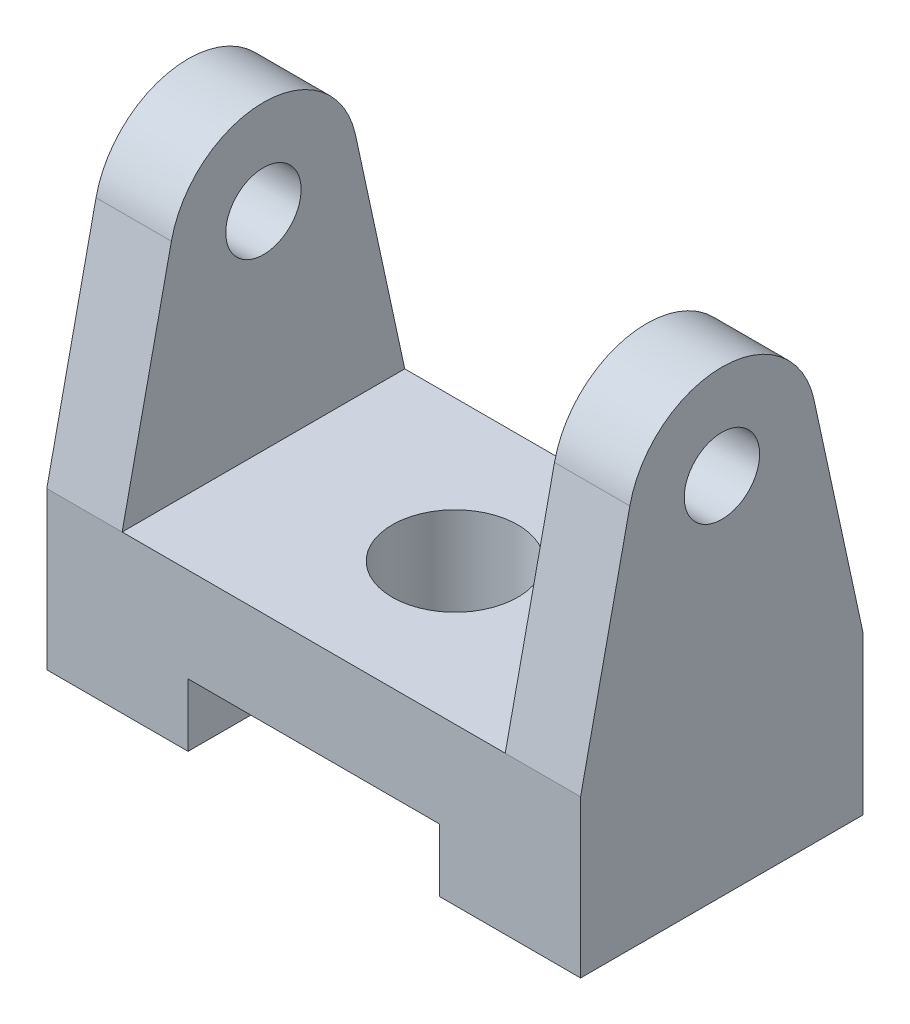
ISO-10303-21;
HEADER;
FILE_DESCRIPTION(('STEP AP214'),'2;1');
FILE_NAME('part.step','',(''),(''),'','','');
FILE_SCHEMA(('AUTOMOTIVE_DESIGN { 1 0 10303 214 1 1 1 1 }'));
ENDSEC;
DATA;
#1=APPLICATION_CONTEXT('core data for automotive mechanical design processes');
#2=APPLICATION_PROTOCOL_DEFINITION('international standard','automotive_design',2000,#1);
#3=PRODUCT_CONTEXT('',#1,'mechanical');
#4=PRODUCT('Part','Part','',(#3));
#5=PRODUCT_RELATED_PRODUCT_CATEGORY('part','',(#4));
#6=PRODUCT_DEFINITION_FORMATION('','',#4);
#7=PRODUCT_DEFINITION_CONTEXT('part definition',#1,'design');
#8=PRODUCT_DEFINITION('design','',#6,#7);
#9=PRODUCT_DEFINITION_SHAPE('','',#8);
#10=(LENGTH_UNIT() NAMED_UNIT(*) SI_UNIT(.MILLI.,.METRE.));
#11=(NAMED_UNIT(*) PLANE_ANGLE_UNIT() SI_UNIT($,.RADIAN.));
#12=(NAMED_UNIT(*) SI_UNIT($,.STERADIAN.) SOLID_ANGLE_UNIT());
#13=UNCERTAINTY_MEASURE_WITH_UNIT(LENGTH_MEASURE(1.E-05),#10,'distance_accuracy_value','');
#14=(GEOMETRIC_REPRESENTATION_CONTEXT(3) GLOBAL_UNCERTAINTY_ASSIGNED_CONTEXT((#13)) GLOBAL_UNIT_ASSIGNED_CONTEXT((#10,
#11,#12)) REPRESENTATION_CONTEXT('',''));
#15=CARTESIAN_POINT('',(0.,0.,0.));
#16=DIRECTION('',(0.,0.,1.));
#17=DIRECTION('',(1.,0.,0.));
#18=AXIS2_PLACEMENT_3D('',#15,#16,#17);
#19=CARTESIAN_POINT('',(-42.5,25.,45.));
#20=DIRECTION('',(0.,-1.,0.));
#21=DIRECTION('',(0.,0.,-1.));
#22=AXIS2_PLACEMENT_3D('',#19,#20,#21);
#23=PLANE('',#22);
#24=CARTESIAN_POINT('',(0.,25.,22.5));
#25=DIRECTION('',(0.,1.,0.));
#26=DIRECTION('',(0.,0.,1.));
#27=AXIS2_PLACEMENT_3D('',#24,#25,#26);
#28=CIRCLE('',#27,10.);
#29=CARTESIAN_POINT('',(0.,25.,32.5));
#30=VERTEX_POINT('',#29);
#31=EDGE_CURVE('E212',#30,#30,#28,.T.);
#32=ORIENTED_EDGE('',*,*,#31,.F.);
#33=EDGE_LOOP('',(#32));
#34=FACE_BOUND('',#33,.T.);
#35=DIRECTION('',(0.,0.,-1.));
#36=VECTOR('',#35,1.);
#37=CARTESIAN_POINT('',(30.5,25.,45.));
#38=LINE('',#37,#36);
#39=CARTESIAN_POINT('',(30.5,25.,45.));
#40=VERTEX_POINT('',#39);
#41=CARTESIAN_POINT('',(30.5,25.,0.));
#42=VERTEX_POINT('',#41);
#43=EDGE_CURVE('E170',#40,#42,#38,.T.);
#44=ORIENTED_EDGE('',*,*,#43,.T.);
#45=DIRECTION('',(-1.,0.,0.));
#46=VECTOR('',#45,1.);
#47=CARTESIAN_POINT('',(-42.5,25.,0.));
#48=LINE('',#47,#46);
#49=CARTESIAN_POINT('',(-30.5,25.,0.));
#50=VERTEX_POINT('',#49);
#51=EDGE_CURVE('E245',#42,#50,#48,.T.);
#52=ORIENTED_EDGE('',*,*,#51,.T.);
#53=DIRECTION('',(0.,0.,1.));
#54=VECTOR('',#53,1.);
#55=CARTESIAN_POINT('',(-30.5,25.,0.));
#56=LINE('',#55,#54);
#57=CARTESIAN_POINT('',(-30.5,25.,45.));
#58=VERTEX_POINT('',#57);
#59=EDGE_CURVE('E192',#50,#58,#56,.T.);
#60=ORIENTED_EDGE('',*,*,#59,.T.);
#61=DIRECTION('',(-1.,0.,0.));
#62=VECTOR('',#61,1.);
#63=CARTESIAN_POINT('',(-42.5,25.,45.));
#64=LINE('',#63,#62);
#65=EDGE_CURVE('E58',#40,#58,#64,.T.);
#66=ORIENTED_EDGE('',*,*,#65,.F.);
#67=EDGE_LOOP('',(#44,#52,#60,#66));
#68=FACE_BOUND('',#67,.T.);
#69=ADVANCED_FACE('F44',(#34,#68),#23,.F.);
#70=CARTESIAN_POINT('',(-42.5,0.,45.));
#71=DIRECTION('',(1.,0.,0.));
#72=DIRECTION('',(0.,0.,-1.));
#73=AXIS2_PLACEMENT_3D('',#70,#71,#72);
#74=PLANE('',#73);
#75=DIRECTION('',(0.,-1.,0.));
#76=VECTOR('',#75,1.);
#77=CARTESIAN_POINT('',(-42.5,0.,0.));
#78=LINE('',#77,#76);
#79=CARTESIAN_POINT('',(-42.5,25.,0.));
#80=VERTEX_POINT('',#79);
#81=CARTESIAN_POINT('',(-42.5,0.,0.));
#82=VERTEX_POINT('',#81);
#83=EDGE_CURVE('E241',#80,#82,#78,.T.);
#84=ORIENTED_EDGE('',*,*,#83,.T.);
#85=DIRECTION('',(0.,0.,-1.));
#86=VECTOR('',#85,1.);
#87=CARTESIAN_POINT('',(-42.5,0.,45.));
#88=LINE('',#87,#86);
#89=CARTESIAN_POINT('',(-42.5,0.,45.));
#90=VERTEX_POINT('',#89);
#91=EDGE_CURVE('E11',#90,#82,#88,.T.);
#92=ORIENTED_EDGE('',*,*,#91,.F.);
#93=DIRECTION('',(0.,-1.,0.));
#94=VECTOR('',#93,1.);
#95=CARTESIAN_POINT('',(-42.5,0.,45.));
#96=LINE('',#95,#94);
#97=CARTESIAN_POINT('',(-42.5,25.,45.));
#98=VERTEX_POINT('',#97);
#99=EDGE_CURVE('E221',#98,#90,#96,.T.);
#100=ORIENTED_EDGE('',*,*,#99,.F.);
#101=DIRECTION('',(0.,0.977312211406396,-0.211803780504361));
#102=VECTOR('',#101,1.);
#103=CARTESIAN_POINT('',(-42.5,25.,45.));
#104=LINE('',#103,#102);
#105=CARTESIAN_POINT('',(-42.5,61.1770567075654,37.159683171096));
#106=VERTEX_POINT('',#105);
#107=EDGE_CURVE('E210',#98,#106,#104,.T.);
#108=ORIENTED_EDGE('',*,*,#107,.T.);
#109=CARTESIAN_POINT('',(-42.5,58.,22.5));
#110=DIRECTION('',(-1.,0.,0.));
#111=DIRECTION('',(0.,0.,1.));
#112=AXIS2_PLACEMENT_3D('',#109,#110,#111);
#113=CIRCLE('',#112,15.);
#114=CARTESIAN_POINT('',(-42.5,61.1770567075654,7.84031682890406));
#115=VERTEX_POINT('',#114);
#116=EDGE_CURVE('E198',#106,#115,#113,.T.);
#117=ORIENTED_EDGE('',*,*,#116,.T.);
#118=DIRECTION('',(0.,-0.977312211406396,-0.211803780504361));
#119=VECTOR('',#118,1.);
#120=CARTESIAN_POINT('',(-42.5,25.,0.));
#121=LINE('',#120,#119);
#122=EDGE_CURVE('E188',#115,#80,#121,.T.);
#123=ORIENTED_EDGE('',*,*,#122,.T.);
#124=EDGE_LOOP('',(#84,#92,#100,#108,#117,#123));
#125=FACE_BOUND('',#124,.T.);
#126=CARTESIAN_POINT('',(-42.5,58.,22.5));
#127=DIRECTION('',(-1.,0.,0.));
#128=DIRECTION('',(0.,0.,1.));
#129=AXIS2_PLACEMENT_3D('',#126,#127,#128);
#130=CIRCLE('',#129,6.00000000000001);
#131=CARTESIAN_POINT('',(-42.5,58.,28.5));
#132=VERTEX_POINT('',#131);
#133=EDGE_CURVE('E184',#132,#132,#130,.T.);
#134=ORIENTED_EDGE('',*,*,#133,.F.);
#135=EDGE_LOOP('',(#134));
#136=FACE_BOUND('',#135,.T.);
#137=ADVANCED_FACE('F297',(#125,#136),#74,.F.);
#138=CARTESIAN_POINT('',(-20.,0.,45.));
#139=DIRECTION('',(0.,1.,0.));
#140=DIRECTION('',(0.,0.,1.));
#141=AXIS2_PLACEMENT_3D('',#138,#139,#140);
#142=PLANE('',#141);
#143=DIRECTION('',(1.,0.,0.));
#144=VECTOR('',#143,1.);
#145=CARTESIAN_POINT('',(-20.,0.,0.));
#146=LINE('',#145,#144);
#147=CARTESIAN_POINT('',(-20.,0.,0.));
#148=VERTEX_POINT('',#147);
#149=EDGE_CURVE('E242',#82,#148,#146,.T.);
#150=ORIENTED_EDGE('',*,*,#149,.T.);
#151=DIRECTION('',(0.,0.,-1.));
#152=VECTOR('',#151,1.);
#153=CARTESIAN_POINT('',(-20.,0.,45.));
#154=LINE('',#153,#152);
#155=CARTESIAN_POINT('',(-20.,0.,45.));
#156=VERTEX_POINT('',#155);
#157=EDGE_CURVE('E52',#156,#148,#154,.T.);
#158=ORIENTED_EDGE('',*,*,#157,.F.);
#159=DIRECTION('',(1.,0.,0.));
#160=VECTOR('',#159,1.);
#161=CARTESIAN_POINT('',(-20.,0.,45.));
#162=LINE('',#161,#160);
#163=EDGE_CURVE('E229',#90,#156,#162,.T.);
#164=ORIENTED_EDGE('',*,*,#163,.F.);
#165=ORIENTED_EDGE('',*,*,#91,.T.);
#166=EDGE_LOOP('',(#150,#158,#164,#165));
#167=FACE_BOUND('',#166,.T.);
#168=ADVANCED_FACE('F300',(#167),#142,.F.);
#169=CARTESIAN_POINT('',(-20.,10.,45.));
#170=DIRECTION('',(-1.,0.,0.));
#171=DIRECTION('',(0.,0.,1.));
#172=AXIS2_PLACEMENT_3D('',#169,#170,#171);
#173=PLANE('',#172);
#174=DIRECTION('',(0.,1.,0.));
#175=VECTOR('',#174,1.);
#176=CARTESIAN_POINT('',(-20.,10.,0.));
#177=LINE('',#176,#175);
#178=CARTESIAN_POINT('',(-20.,10.,0.));
#179=VERTEX_POINT('',#178);
#180=EDGE_CURVE('E250',#148,#179,#177,.T.);
#181=ORIENTED_EDGE('',*,*,#180,.T.);
#182=DIRECTION('',(0.,0.,-1.));
#183=VECTOR('',#182,1.);
#184=CARTESIAN_POINT('',(-20.,10.,45.));
#185=LINE('',#184,#183);
#186=CARTESIAN_POINT('',(-20.,10.,45.));
#187=VERTEX_POINT('',#186);
#188=EDGE_CURVE('E264',#187,#179,#185,.T.);
#189=ORIENTED_EDGE('',*,*,#188,.F.);
#190=DIRECTION('',(0.,1.,0.));
#191=VECTOR('',#190,1.);
#192=CARTESIAN_POINT('',(-20.,10.,45.));
#193=LINE('',#192,#191);
#194=EDGE_CURVE('E230',#156,#187,#193,.T.);
#195=ORIENTED_EDGE('',*,*,#194,.F.);
#196=ORIENTED_EDGE('',*,*,#157,.T.);
#197=EDGE_LOOP('',(#181,#189,#195,#196));
#198=FACE_BOUND('',#197,.T.);
#199=ADVANCED_FACE('F272',(#198),#173,.F.);
#200=CARTESIAN_POINT('',(20.,10.,45.));
#201=DIRECTION('',(0.,1.,0.));
#202=DIRECTION('',(0.,0.,1.));
#203=AXIS2_PLACEMENT_3D('',#200,#201,#202);
#204=PLANE('',#203);
#205=CARTESIAN_POINT('',(0.,10.,22.5));
#206=DIRECTION('',(0.,1.,0.));
#207=DIRECTION('',(0.,0.,1.));
#208=AXIS2_PLACEMENT_3D('',#205,#206,#207);
#209=CIRCLE('',#208,10.);
#210=CARTESIAN_POINT('',(0.,10.,32.5));
#211=VERTEX_POINT('',#210);
#212=EDGE_CURVE('E48',#211,#211,#209,.T.);
#213=ORIENTED_EDGE('',*,*,#212,.T.);
#214=EDGE_LOOP('',(#213));
#215=FACE_BOUND('',#214,.T.);
#216=DIRECTION('',(1.,0.,0.));
#217=VECTOR('',#216,1.);
#218=CARTESIAN_POINT('',(20.,10.,0.));
#219=LINE('',#218,#217);
#220=CARTESIAN_POINT('',(20.,10.,0.));
#221=VERTEX_POINT('',#220);
#222=EDGE_CURVE('E249',#179,#221,#219,.T.);
#223=ORIENTED_EDGE('',*,*,#222,.T.);
#224=DIRECTION('',(0.,0.,-1.));
#225=VECTOR('',#224,1.);
#226=CARTESIAN_POINT('',(20.,10.,45.));
#227=LINE('',#226,#225);
#228=CARTESIAN_POINT('',(20.,10.,45.));
#229=VERTEX_POINT('',#228);
#230=EDGE_CURVE('E265',#229,#221,#227,.T.);
#231=ORIENTED_EDGE('',*,*,#230,.F.);
#232=DIRECTION('',(1.,0.,0.));
#233=VECTOR('',#232,1.);
#234=CARTESIAN_POINT('',(20.,10.,45.));
#235=LINE('',#234,#233);
#236=EDGE_CURVE('E227',#187,#229,#235,.T.);
#237=ORIENTED_EDGE('',*,*,#236,.F.);
#238=ORIENTED_EDGE('',*,*,#188,.T.);
#239=EDGE_LOOP('',(#223,#231,#237,#238));
#240=FACE_BOUND('',#239,.T.);
#241=ADVANCED_FACE('F290',(#215,#240),#204,.F.);
#242=CARTESIAN_POINT('',(20.,0.,45.));
#243=DIRECTION('',(1.,0.,0.));
#244=DIRECTION('',(0.,0.,-1.));
#245=AXIS2_PLACEMENT_3D('',#242,#243,#244);
#246=PLANE('',#245);
#247=DIRECTION('',(0.,-1.,0.));
#248=VECTOR('',#247,1.);
#249=CARTESIAN_POINT('',(20.,0.,0.));
#250=LINE('',#249,#248);
#251=CARTESIAN_POINT('',(20.,0.,0.));
#252=VERTEX_POINT('',#251);
#253=EDGE_CURVE('E253',#221,#252,#250,.T.);
#254=ORIENTED_EDGE('',*,*,#253,.T.);
#255=DIRECTION('',(0.,0.,-1.));
#256=VECTOR('',#255,1.);
#257=CARTESIAN_POINT('',(20.,0.,45.));
#258=LINE('',#257,#256);
#259=CARTESIAN_POINT('',(20.,0.,45.));
#260=VERTEX_POINT('',#259);
#261=EDGE_CURVE('E259',#260,#252,#258,.T.);
#262=ORIENTED_EDGE('',*,*,#261,.F.);
#263=DIRECTION('',(0.,-1.,0.));
#264=VECTOR('',#263,1.);
#265=CARTESIAN_POINT('',(20.,0.,45.));
#266=LINE('',#265,#264);
#267=EDGE_CURVE('E235',#229,#260,#266,.T.);
#268=ORIENTED_EDGE('',*,*,#267,.F.);
#269=ORIENTED_EDGE('',*,*,#230,.T.);
#270=EDGE_LOOP('',(#254,#262,#268,#269));
#271=FACE_BOUND('',#270,.T.);
#272=ADVANCED_FACE('F292',(#271),#246,.F.);
#273=CARTESIAN_POINT('',(42.5,0.,45.));
#274=DIRECTION('',(0.,1.,0.));
#275=DIRECTION('',(0.,0.,1.));
#276=AXIS2_PLACEMENT_3D('',#273,#274,#275);
#277=PLANE('',#276);
#278=DIRECTION('',(1.,0.,0.));
#279=VECTOR('',#278,1.);
#280=CARTESIAN_POINT('',(42.5,0.,0.));
#281=LINE('',#280,#279);
#282=CARTESIAN_POINT('',(42.5,0.,0.));
#283=VERTEX_POINT('',#282);
#284=EDGE_CURVE('E251',#252,#283,#281,.T.);
#285=ORIENTED_EDGE('',*,*,#284,.T.);
#286=DIRECTION('',(0.,0.,-1.));
#287=VECTOR('',#286,1.);
#288=CARTESIAN_POINT('',(42.5,0.,45.));
#289=LINE('',#288,#287);
#290=CARTESIAN_POINT('',(42.5,0.,45.));
#291=VERTEX_POINT('',#290);
#292=EDGE_CURVE('E236',#291,#283,#289,.T.);
#293=ORIENTED_EDGE('',*,*,#292,.F.);
#294=DIRECTION('',(1.,0.,0.));
#295=VECTOR('',#294,1.);
#296=CARTESIAN_POINT('',(42.5,0.,45.));
#297=LINE('',#296,#295);
#298=EDGE_CURVE('E234',#260,#291,#297,.T.);
#299=ORIENTED_EDGE('',*,*,#298,.F.);
#300=ORIENTED_EDGE('',*,*,#261,.T.);
#301=EDGE_LOOP('',(#285,#293,#299,#300));
#302=FACE_BOUND('',#301,.T.);
#303=ADVANCED_FACE('F355',(#302),#277,.F.);
#304=CARTESIAN_POINT('',(42.5,25.,45.));
#305=DIRECTION('',(-1.,0.,0.));
#306=DIRECTION('',(0.,0.,1.));
#307=AXIS2_PLACEMENT_3D('',#304,#305,#306);
#308=PLANE('',#307);
#309=DIRECTION('',(0.,1.,0.));
#310=VECTOR('',#309,1.);
#311=CARTESIAN_POINT('',(42.5,25.,0.));
#312=LINE('',#311,#310);
#313=CARTESIAN_POINT('',(42.5,25.,0.));
#314=VERTEX_POINT('',#313);
#315=EDGE_CURVE('E254',#283,#314,#312,.T.);
#316=ORIENTED_EDGE('',*,*,#315,.T.);
#317=DIRECTION('',(0.,0.977312211406396,0.211803780504361));
#318=VECTOR('',#317,1.);
#319=CARTESIAN_POINT('',(42.5,25.,0.));
#320=LINE('',#319,#318);
#321=CARTESIAN_POINT('',(42.5,61.1770567075654,7.84031682890406));
#322=VERTEX_POINT('',#321);
#323=EDGE_CURVE('E168',#314,#322,#320,.T.);
#324=ORIENTED_EDGE('',*,*,#323,.T.);
#325=CARTESIAN_POINT('',(42.5,58.,22.5));
#326=DIRECTION('',(1.,0.,0.));
#327=DIRECTION('',(0.,0.,-1.));
#328=AXIS2_PLACEMENT_3D('',#325,#326,#327);
#329=CIRCLE('',#328,15.);
#330=CARTESIAN_POINT('',(42.5,61.1770567075654,37.159683171096));
#331=VERTEX_POINT('',#330);
#332=EDGE_CURVE('E177',#322,#331,#329,.T.);
#333=ORIENTED_EDGE('',*,*,#332,.T.);
#334=DIRECTION('',(0.,-0.977312211406396,0.211803780504361));
#335=VECTOR('',#334,1.);
#336=CARTESIAN_POINT('',(42.5,61.1770567075654,37.159683171096));
#337=LINE('',#336,#335);
#338=CARTESIAN_POINT('',(42.5,25.,45.));
#339=VERTEX_POINT('',#338);
#340=EDGE_CURVE('E155',#331,#339,#337,.T.);
#341=ORIENTED_EDGE('',*,*,#340,.T.);
#342=DIRECTION('',(0.,1.,0.));
#343=VECTOR('',#342,1.);
#344=CARTESIAN_POINT('',(42.5,25.,45.));
#345=LINE('',#344,#343);
#346=EDGE_CURVE('E237',#291,#339,#345,.T.);
#347=ORIENTED_EDGE('',*,*,#346,.F.);
#348=ORIENTED_EDGE('',*,*,#292,.T.);
#349=EDGE_LOOP('',(#316,#324,#333,#341,#347,#348));
#350=FACE_BOUND('',#349,.T.);
#351=CARTESIAN_POINT('',(42.5,58.,22.5));
#352=DIRECTION('',(1.,0.,0.));
#353=DIRECTION('',(0.,0.,-1.));
#354=AXIS2_PLACEMENT_3D('',#351,#352,#353);
#355=CIRCLE('',#354,6.00000000000001);
#356=CARTESIAN_POINT('',(42.5,58.,16.5));
#357=VERTEX_POINT('',#356);
#358=EDGE_CURVE('E172',#357,#357,#355,.T.);
#359=ORIENTED_EDGE('',*,*,#358,.F.);
#360=EDGE_LOOP('',(#359));
#361=FACE_BOUND('',#360,.T.);
#362=ADVANCED_FACE('F358',(#350,#361),#308,.F.);
#363=CARTESIAN_POINT('',(0.,0.,45.));
#364=DIRECTION('',(0.,0.,-1.));
#365=DIRECTION('',(-1.,0.,0.));
#366=AXIS2_PLACEMENT_3D('',#363,#364,#365);
#367=PLANE('',#366);
#368=EDGE_CURVE('E225',#339,#40,#64,.T.);
#369=ORIENTED_EDGE('',*,*,#368,.T.);
#370=ORIENTED_EDGE('',*,*,#65,.T.);
#371=DIRECTION('',(-1.,0.,0.));
#372=VECTOR('',#371,1.);
#373=CARTESIAN_POINT('',(-30.5,25.,45.));
#374=LINE('',#373,#372);
#375=EDGE_CURVE('E220',#58,#98,#374,.T.);
#376=ORIENTED_EDGE('',*,*,#375,.T.);
#377=ORIENTED_EDGE('',*,*,#99,.T.);
#378=ORIENTED_EDGE('',*,*,#163,.T.);
#379=ORIENTED_EDGE('',*,*,#194,.T.);
#380=ORIENTED_EDGE('',*,*,#236,.T.);
#381=ORIENTED_EDGE('',*,*,#267,.T.);
#382=ORIENTED_EDGE('',*,*,#298,.T.);
#383=ORIENTED_EDGE('',*,*,#346,.T.);
#384=EDGE_LOOP('',(#369,#370,#376,#377,#378,#379,#380,#381,#382,#383));
#385=FACE_BOUND('',#384,.T.);
#386=ADVANCED_FACE('F294',(#385),#367,.F.);
#387=CARTESIAN_POINT('',(0.,0.,0.));
#388=DIRECTION('',(0.,0.,-1.));
#389=DIRECTION('',(-1.,0.,0.));
#390=AXIS2_PLACEMENT_3D('',#387,#388,#389);
#391=PLANE('',#390);
#392=EDGE_CURVE('E239',#314,#42,#48,.T.);
#393=ORIENTED_EDGE('',*,*,#392,.F.);
#394=ORIENTED_EDGE('',*,*,#315,.F.);
#395=ORIENTED_EDGE('',*,*,#284,.F.);
#396=ORIENTED_EDGE('',*,*,#253,.F.);
#397=ORIENTED_EDGE('',*,*,#222,.F.);
#398=ORIENTED_EDGE('',*,*,#180,.F.);
#399=ORIENTED_EDGE('',*,*,#149,.F.);
#400=ORIENTED_EDGE('',*,*,#83,.F.);
#401=DIRECTION('',(-1.,0.,0.));
#402=VECTOR('',#401,1.);
#403=CARTESIAN_POINT('',(-30.5,25.,0.));
#404=LINE('',#403,#402);
#405=EDGE_CURVE('E204',#50,#80,#404,.T.);
#406=ORIENTED_EDGE('',*,*,#405,.F.);
#407=ORIENTED_EDGE('',*,*,#51,.F.);
#408=EDGE_LOOP('',(#393,#394,#395,#396,#397,#398,#399,#400,#406,#407));
#409=FACE_BOUND('',#408,.T.);
#410=ADVANCED_FACE('F284',(#409),#391,.T.);
#411=CARTESIAN_POINT('',(0.,-20.,22.5));
#412=DIRECTION('',(0.,1.,0.));
#413=DIRECTION('',(0.,0.,1.));
#414=AXIS2_PLACEMENT_3D('',#411,#412,#413);
#415=CYLINDRICAL_SURFACE('',#414,10.);
#416=CARTESIAN_POINT('',(0.,25.,32.5));
#417=CARTESIAN_POINT('',(0.,24.84375,32.5));
#418=CARTESIAN_POINT('',(0.,24.6875,32.5));
#419=CARTESIAN_POINT('',(0.,24.375,32.5));
#420=CARTESIAN_POINT('',(0.,24.21875,32.5));
#421=CARTESIAN_POINT('',(0.,23.90625,32.5));
#422=CARTESIAN_POINT('',(0.,23.75,32.5));
#423=CARTESIAN_POINT('',(0.,23.4375,32.5));
#424=CARTESIAN_POINT('',(0.,23.28125,32.5));
#425=CARTESIAN_POINT('',(0.,22.96875,32.5));
#426=CARTESIAN_POINT('',(0.,22.8125,32.5));
#427=CARTESIAN_POINT('',(0.,22.5,32.5));
#428=CARTESIAN_POINT('',(0.,22.34375,32.5));
#429=CARTESIAN_POINT('',(0.,22.03125,32.5));
#430=CARTESIAN_POINT('',(0.,21.875,32.5));
#431=CARTESIAN_POINT('',(0.,21.5625,32.5));
#432=CARTESIAN_POINT('',(0.,21.40625,32.5));
#433=CARTESIAN_POINT('',(0.,21.09375,32.5));
#434=CARTESIAN_POINT('',(0.,20.9375,32.5));
#435=CARTESIAN_POINT('',(0.,20.625,32.5));
#436=CARTESIAN_POINT('',(0.,20.46875,32.5));
#437=CARTESIAN_POINT('',(0.,20.15625,32.5));
#438=CARTESIAN_POINT('',(0.,20.,32.5));
#439=CARTESIAN_POINT('',(0.,19.6875,32.5));
#440=CARTESIAN_POINT('',(0.,19.53125,32.5));
#441=CARTESIAN_POINT('',(0.,19.21875,32.5));
#442=CARTESIAN_POINT('',(0.,19.0625,32.5));
#443=CARTESIAN_POINT('',(0.,18.75,32.5));
#444=CARTESIAN_POINT('',(0.,18.59375,32.5));
#445=CARTESIAN_POINT('',(0.,18.28125,32.5));
#446=CARTESIAN_POINT('',(0.,18.125,32.5));
#447=CARTESIAN_POINT('',(0.,17.8125,32.5));
#448=CARTESIAN_POINT('',(0.,17.65625,32.5));
#449=CARTESIAN_POINT('',(0.,17.34375,32.5));
#450=CARTESIAN_POINT('',(0.,17.1875,32.5));
#451=CARTESIAN_POINT('',(0.,16.875,32.5));
#452=CARTESIAN_POINT('',(0.,16.71875,32.5));
#453=CARTESIAN_POINT('',(0.,16.40625,32.5));
#454=CARTESIAN_POINT('',(0.,16.25,32.5));
#455=CARTESIAN_POINT('',(0.,15.9375,32.5));
#456=CARTESIAN_POINT('',(0.,15.78125,32.5));
#457=CARTESIAN_POINT('',(0.,15.46875,32.5));
#458=CARTESIAN_POINT('',(0.,15.3125,32.5));
#459=CARTESIAN_POINT('',(0.,15.,32.5));
#460=CARTESIAN_POINT('',(0.,14.84375,32.5));
#461=CARTESIAN_POINT('',(0.,14.53125,32.5));
#462=CARTESIAN_POINT('',(0.,14.375,32.5));
#463=CARTESIAN_POINT('',(0.,14.0625,32.5));
#464=CARTESIAN_POINT('',(0.,13.90625,32.5));
#465=CARTESIAN_POINT('',(0.,13.59375,32.5));
#466=CARTESIAN_POINT('',(0.,13.4375,32.5));
#467=CARTESIAN_POINT('',(0.,13.125,32.5));
#468=CARTESIAN_POINT('',(0.,12.96875,32.5));
#469=CARTESIAN_POINT('',(0.,12.65625,32.5));
#470=CARTESIAN_POINT('',(0.,12.5,32.5));
#471=CARTESIAN_POINT('',(0.,12.1875,32.5));
#472=CARTESIAN_POINT('',(0.,12.03125,32.5));
#473=CARTESIAN_POINT('',(0.,11.71875,32.5));
#474=CARTESIAN_POINT('',(0.,11.5625,32.5));
#475=CARTESIAN_POINT('',(0.,11.25,32.5));
#476=CARTESIAN_POINT('',(0.,11.09375,32.5));
#477=CARTESIAN_POINT('',(0.,10.78125,32.5));
#478=CARTESIAN_POINT('',(0.,10.625,32.5));
#479=CARTESIAN_POINT('',(0.,10.3125,32.5));
#480=CARTESIAN_POINT('',(0.,10.15625,32.5));
#481=CARTESIAN_POINT('',(0.,10.,32.5));
#482=B_SPLINE_CURVE_WITH_KNOTS('',3,(#416,#417,#418,#419,#420,#421,#422,#423,#424,#425,#426,
#427,#428,#429,#430,#431,#432,#433,#434,#435,#436,#437,#438,#439,#440,#441,#442,#443,#444,#445,
#446,#447,#448,#449,#450,#451,#452,#453,#454,#455,#456,#457,#458,#459,#460,#461,#462,#463,#464,
#465,#466,#467,#468,#469,#470,#471,#472,#473,#474,#475,#476,#477,#478,#479,#480,#481),
.UNSPECIFIED.,.F.,.F.,(4,2,2,2,2,2,2,2,2,2,2,2,2,2,2,2,2,2,2,2,2,2,2,2,2,2,2,2,2,2,2,2,4),(0.,
0.468749999999997,0.937500000000001,1.40625,1.875,2.34375,2.8125,3.28125,3.75,4.21875,4.6875,
5.15625,5.625,6.09375,6.5625,7.03125,7.5,7.96875,8.4375,8.90625,9.375,9.84375,10.3125,10.78125,
11.25,11.71875,12.1875,12.65625,13.125,13.59375,14.0625,14.53125,15.),.UNSPECIFIED.);
#483=EDGE_CURVE('BSEAM321',#30,#211,#482,.T.);
#484=ORIENTED_EDGE('',*,*,#31,.T.);
#485=ORIENTED_EDGE('',*,*,#212,.F.);
#486=ORIENTED_EDGE('',*,*,#483,.T.);
#487=ORIENTED_EDGE('',*,*,#483,.F.);
#488=EDGE_LOOP('',(#484,#486,#485,#487));
#489=FACE_BOUND('',#488,.T.);
#490=ADVANCED_FACE('F321',(#489),#415,.F.);
#491=CARTESIAN_POINT('',(-30.5,25.,0.));
#492=DIRECTION('',(0.,0.211803780504361,-0.977312211406396));
#493=DIRECTION('',(0.,0.977312211406396,0.211803780504361));
#494=AXIS2_PLACEMENT_3D('',#491,#492,#493);
#495=PLANE('',#494);
#496=ORIENTED_EDGE('',*,*,#122,.F.);
#497=DIRECTION('',(-1.,0.,0.));
#498=VECTOR('',#497,1.);
#499=CARTESIAN_POINT('',(-30.5,61.1770567075654,7.84031682890406));
#500=LINE('',#499,#498);
#501=CARTESIAN_POINT('',(-30.5,61.1770567075654,7.84031682890406));
#502=VERTEX_POINT('',#501);
#503=EDGE_CURVE('E215',#502,#115,#500,.T.);
#504=ORIENTED_EDGE('',*,*,#503,.F.);
#505=DIRECTION('',(0.,-0.977312211406396,-0.211803780504361));
#506=VECTOR('',#505,1.);
#507=CARTESIAN_POINT('',(-30.5,25.,0.));
#508=LINE('',#507,#506);
#509=EDGE_CURVE('E195',#502,#50,#508,.T.);
#510=ORIENTED_EDGE('',*,*,#509,.T.);
#511=ORIENTED_EDGE('',*,*,#405,.T.);
#512=EDGE_LOOP('',(#496,#504,#510,#511));
#513=FACE_BOUND('',#512,.T.);
#514=ADVANCED_FACE('F302',(#513),#495,.T.);
#515=CARTESIAN_POINT('',(-30.5,58.,22.5));
#516=DIRECTION('',(-1.,0.,0.));
#517=DIRECTION('',(0.,0.,1.));
#518=AXIS2_PLACEMENT_3D('',#515,#516,#517);
#519=CYLINDRICAL_SURFACE('',#518,15.);
#520=ORIENTED_EDGE('',*,*,#116,.F.);
#521=DIRECTION('',(-1.,0.,0.));
#522=VECTOR('',#521,1.);
#523=CARTESIAN_POINT('',(-30.5,61.1770567075654,37.159683171096));
#524=LINE('',#523,#522);
#525=CARTESIAN_POINT('',(-30.5,61.1770567075654,37.159683171096));
#526=VERTEX_POINT('',#525);
#527=EDGE_CURVE('E214',#526,#106,#524,.T.);
#528=ORIENTED_EDGE('',*,*,#527,.F.);
#529=CARTESIAN_POINT('',(-30.5,58.,22.5));
#530=DIRECTION('',(-1.,0.,0.));
#531=DIRECTION('',(0.,0.,1.));
#532=AXIS2_PLACEMENT_3D('',#529,#530,#531);
#533=CIRCLE('',#532,15.);
#534=EDGE_CURVE('E203',#526,#502,#533,.T.);
#535=ORIENTED_EDGE('',*,*,#534,.T.);
#536=ORIENTED_EDGE('',*,*,#503,.T.);
#537=EDGE_LOOP('',(#520,#528,#535,#536));
#538=FACE_BOUND('',#537,.T.);
#539=ADVANCED_FACE('F311',(#538),#519,.T.);
#540=CARTESIAN_POINT('',(-30.5,25.,45.));
#541=DIRECTION('',(0.,0.211803780504361,0.977312211406396));
#542=DIRECTION('',(0.,-0.977312211406396,0.211803780504361));
#543=AXIS2_PLACEMENT_3D('',#540,#541,#542);
#544=PLANE('',#543);
#545=ORIENTED_EDGE('',*,*,#107,.F.);
#546=ORIENTED_EDGE('',*,*,#375,.F.);
#547=DIRECTION('',(0.,0.977312211406396,-0.211803780504361));
#548=VECTOR('',#547,1.);
#549=CARTESIAN_POINT('',(-30.5,25.,45.));
#550=LINE('',#549,#548);
#551=EDGE_CURVE('E196',#58,#526,#550,.T.);
#552=ORIENTED_EDGE('',*,*,#551,.T.);
#553=ORIENTED_EDGE('',*,*,#527,.T.);
#554=EDGE_LOOP('',(#545,#546,#552,#553));
#555=FACE_BOUND('',#554,.T.);
#556=ADVANCED_FACE('F316',(#555),#544,.T.);
#557=CARTESIAN_POINT('',(-30.5,58.,22.5));
#558=DIRECTION('',(-1.,0.,0.));
#559=DIRECTION('',(0.,0.,1.));
#560=AXIS2_PLACEMENT_3D('',#557,#558,#559);
#561=PLANE('',#560);
#562=CARTESIAN_POINT('',(-30.5,58.,22.5));
#563=DIRECTION('',(-1.,0.,0.));
#564=DIRECTION('',(0.,0.,1.));
#565=AXIS2_PLACEMENT_3D('',#562,#563,#564);
#566=CIRCLE('',#565,6.00000000000001);
#567=CARTESIAN_POINT('',(-30.5,58.,28.5));
#568=VERTEX_POINT('',#567);
#569=EDGE_CURVE('E189',#568,#568,#566,.T.);
#570=ORIENTED_EDGE('',*,*,#569,.T.);
#571=EDGE_LOOP('',(#570));
#572=FACE_BOUND('',#571,.T.);
#573=ORIENTED_EDGE('',*,*,#509,.F.);
#574=ORIENTED_EDGE('',*,*,#534,.F.);
#575=ORIENTED_EDGE('',*,*,#551,.F.);
#576=ORIENTED_EDGE('',*,*,#59,.F.);
#577=EDGE_LOOP('',(#573,#574,#575,#576));
#578=FACE_BOUND('',#577,.T.);
#579=ADVANCED_FACE('F309',(#572,#578),#561,.F.);
#580=CARTESIAN_POINT('',(-30.5,58.,22.5));
#581=DIRECTION('',(-1.,0.,0.));
#582=DIRECTION('',(0.,0.,1.));
#583=AXIS2_PLACEMENT_3D('',#580,#581,#582);
#584=CYLINDRICAL_SURFACE('',#583,6.00000000000001);
#585=ORIENTED_EDGE('',*,*,#569,.F.);
#586=EDGE_LOOP('',(#585));
#587=FACE_BOUND('',#586,.T.);
#588=ORIENTED_EDGE('',*,*,#133,.T.);
#589=EDGE_LOOP('',(#588));
#590=FACE_BOUND('',#589,.T.);
#591=ADVANCED_FACE('F377',(#587,#590),#584,.F.);
#592=CARTESIAN_POINT('',(30.5,58.,22.5));
#593=DIRECTION('',(1.,0.,0.));
#594=DIRECTION('',(0.,0.,-1.));
#595=AXIS2_PLACEMENT_3D('',#592,#593,#594);
#596=CYLINDRICAL_SURFACE('',#595,15.);
#597=ORIENTED_EDGE('',*,*,#332,.F.);
#598=DIRECTION('',(1.,0.,0.));
#599=VECTOR('',#598,1.);
#600=CARTESIAN_POINT('',(30.5,61.1770567075654,7.84031682890406));
#601=LINE('',#600,#599);
#602=CARTESIAN_POINT('',(30.5,61.1770567075654,7.84031682890406));
#603=VERTEX_POINT('',#602);
#604=EDGE_CURVE('E160',#603,#322,#601,.T.);
#605=ORIENTED_EDGE('',*,*,#604,.F.);
#606=CARTESIAN_POINT('',(30.5,58.,22.5));
#607=DIRECTION('',(1.,0.,0.));
#608=DIRECTION('',(0.,0.,-1.));
#609=AXIS2_PLACEMENT_3D('',#606,#607,#608);
#610=CIRCLE('',#609,15.);
#611=CARTESIAN_POINT('',(30.5,61.1770567075654,37.159683171096));
#612=VERTEX_POINT('',#611);
#613=EDGE_CURVE('E164',#603,#612,#610,.T.);
#614=ORIENTED_EDGE('',*,*,#613,.T.);
#615=DIRECTION('',(1.,0.,0.));
#616=VECTOR('',#615,1.);
#617=CARTESIAN_POINT('',(30.5,61.1770567075654,37.159683171096));
#618=LINE('',#617,#616);
#619=EDGE_CURVE('E148',#612,#331,#618,.T.);
#620=ORIENTED_EDGE('',*,*,#619,.T.);
#621=EDGE_LOOP('',(#597,#605,#614,#620));
#622=FACE_BOUND('',#621,.T.);
#623=ADVANCED_FACE('F166',(#622),#596,.T.);
#624=CARTESIAN_POINT('',(30.5,25.,0.));
#625=DIRECTION('',(0.,0.211803780504361,-0.977312211406396));
#626=DIRECTION('',(0.,0.977312211406396,0.211803780504361));
#627=AXIS2_PLACEMENT_3D('',#624,#625,#626);
#628=PLANE('',#627);
#629=ORIENTED_EDGE('',*,*,#323,.F.);
#630=ORIENTED_EDGE('',*,*,#392,.T.);
#631=DIRECTION('',(0.,0.977312211406396,0.211803780504361));
#632=VECTOR('',#631,1.);
#633=CARTESIAN_POINT('',(30.5,25.,0.));
#634=LINE('',#633,#632);
#635=EDGE_CURVE('E158',#42,#603,#634,.T.);
#636=ORIENTED_EDGE('',*,*,#635,.T.);
#637=ORIENTED_EDGE('',*,*,#604,.T.);
#638=EDGE_LOOP('',(#629,#630,#636,#637));
#639=FACE_BOUND('',#638,.T.);
#640=ADVANCED_FACE('F378',(#639),#628,.T.);
#641=CARTESIAN_POINT('',(30.5,61.1770567075654,37.159683171096));
#642=DIRECTION('',(0.,0.211803780504361,0.977312211406396));
#643=DIRECTION('',(0.,-0.977312211406396,0.211803780504361));
#644=AXIS2_PLACEMENT_3D('',#641,#642,#643);
#645=PLANE('',#644);
#646=ORIENTED_EDGE('',*,*,#340,.F.);
#647=ORIENTED_EDGE('',*,*,#619,.F.);
#648=DIRECTION('',(0.,-0.977312211406396,0.211803780504361));
#649=VECTOR('',#648,1.);
#650=CARTESIAN_POINT('',(30.5,61.1770567075654,37.159683171096));
#651=LINE('',#650,#649);
#652=EDGE_CURVE('E147',#612,#40,#651,.T.);
#653=ORIENTED_EDGE('',*,*,#652,.T.);
#654=ORIENTED_EDGE('',*,*,#368,.F.);
#655=EDGE_LOOP('',(#646,#647,#653,#654));
#656=FACE_BOUND('',#655,.T.);
#657=ADVANCED_FACE('F146',(#656),#645,.T.);
#658=CARTESIAN_POINT('',(30.5,58.,22.5));
#659=DIRECTION('',(1.,0.,0.));
#660=DIRECTION('',(0.,0.,-1.));
#661=AXIS2_PLACEMENT_3D('',#658,#659,#660);
#662=PLANE('',#661);
#663=CARTESIAN_POINT('',(30.5,58.,22.5));
#664=DIRECTION('',(1.,0.,0.));
#665=DIRECTION('',(0.,0.,-1.));
#666=AXIS2_PLACEMENT_3D('',#663,#664,#665);
#667=CIRCLE('',#666,6.00000000000001);
#668=CARTESIAN_POINT('',(30.5,58.,16.5));
#669=VERTEX_POINT('',#668);
#670=EDGE_CURVE('E185',#669,#669,#667,.T.);
#671=ORIENTED_EDGE('',*,*,#670,.T.);
#672=EDGE_LOOP('',(#671));
#673=FACE_BOUND('',#672,.T.);
#674=ORIENTED_EDGE('',*,*,#613,.F.);
#675=ORIENTED_EDGE('',*,*,#635,.F.);
#676=ORIENTED_EDGE('',*,*,#43,.F.);
#677=ORIENTED_EDGE('',*,*,#652,.F.);
#678=EDGE_LOOP('',(#674,#675,#676,#677));
#679=FACE_BOUND('',#678,.T.);
#680=ADVANCED_FACE('F162',(#673,#679),#662,.F.);
#681=CARTESIAN_POINT('',(30.5,58.,22.5));
#682=DIRECTION('',(1.,0.,0.));
#683=DIRECTION('',(0.,0.,-1.));
#684=AXIS2_PLACEMENT_3D('',#681,#682,#683);
#685=CYLINDRICAL_SURFACE('',#684,6.00000000000001);
#686=ORIENTED_EDGE('',*,*,#670,.F.);
#687=EDGE_LOOP('',(#686));
#688=FACE_BOUND('',#687,.T.);
#689=ORIENTED_EDGE('',*,*,#358,.T.);
#690=EDGE_LOOP('',(#689));
#691=FACE_BOUND('',#690,.T.);
#692=ADVANCED_FACE('F405',(#688,#691),#685,.F.);
#693=CLOSED_SHELL('',(#69,#137,#168,#199,#241,#272,#303,#362,#386,#410,#490,#514,#539,#556,#579,
#591,#623,#640,#657,#680,#692));
#694=MANIFOLD_SOLID_BREP('B2',#693);
#695=ADVANCED_BREP_SHAPE_REPRESENTATION('',(#18,#694),#14);
#696=SHAPE_DEFINITION_REPRESENTATION(#9,#695);
ENDSEC;
END-ISO-10303-21;
